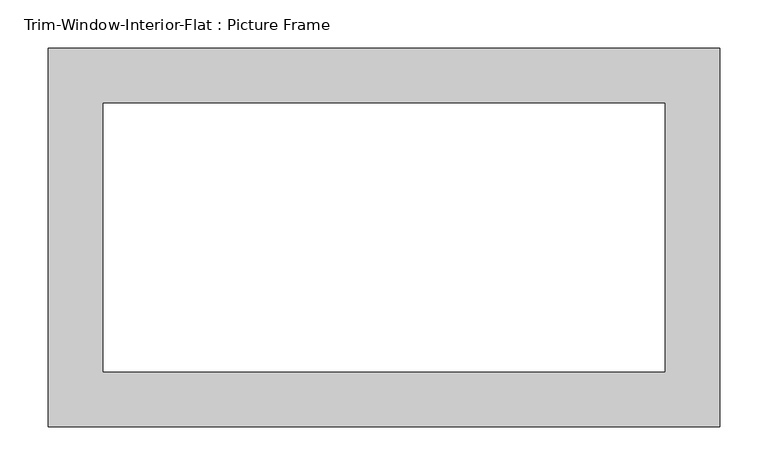
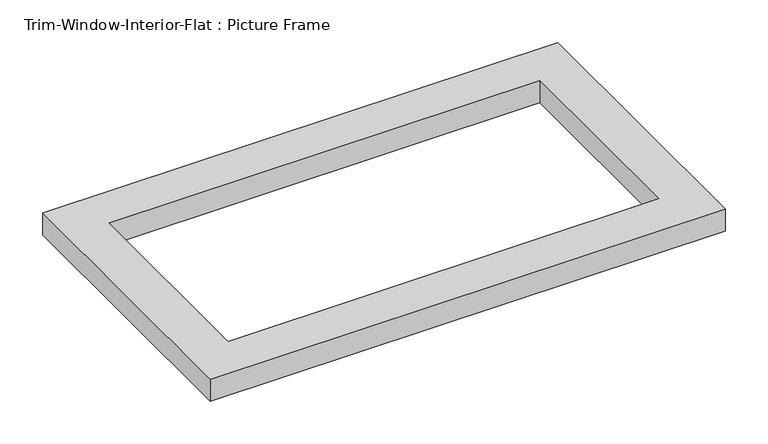
"""IFC4 building model written with IfcOpenShell, lengths in millimetres: proxy geometry, Trim-Window-Interior-Flat : Picture Frame."""

from ifc_helpers import new_model, si_unit, origin, origin_with_axes, place, context, project, spatial, polyline, outline, extrude, source, transform, mapped, element, save


def trim_window_interior_flat_picture_frame_d1e4ee8f(model_context):
    return source(origin(), model_context, "Body", "SweptSolid", [
        extrude(outline(polyline([(349.25, 44.45), (349.25, -349.25), (-349.25, -349.25), (-349.25, 44.45), (349.25, 44.45)]), holes=[polyline([(292.1, -12.7), (-292.1, -12.7), (-292.1, -292.1), (292.1, -292.1), (292.1, -12.7)])]), origin_with_axes(), (0.0, 0.0, 1.0), 31.75),
    ])


if __name__ == "__main__":
    model = new_model("IFC4")
    model_context = context("Model", 3, world=origin())
    ifc_project = project(units=[si_unit("LENGTHUNIT", "METRE", prefix="MILLI")], contexts=[model_context])
    site = spatial("IfcSite", under=ifc_project)
    building = spatial("IfcBuilding", under=site)
    placement = place(None, origin())
    trim_window_interior_flat_picture_frame_shape = trim_window_interior_flat_picture_frame_d1e4ee8f(model_context)
    element("IfcBuildingElementProxy", 1, Name="Trim-Window-Interior-Flat : Picture Frame", ObjectType="Trim-Window-Interior-Flat : Picture Frame", at=placement, inside=building, context=model_context, shape_type="MappedRepresentation", body=[
        mapped(trim_window_interior_flat_picture_frame_shape, transform((0.0, 0.0, 0.0), x_axis=(1.0, 0.0, 0.0), y_axis=(0.0, 1.0, 0.0), z_axis=(0.0, 0.0, 1.0))),
    ])
    save(model, "model.ifc")

# Revit data of these elements
# Type "Trim-Window-Interior-Flat : Picture Frame"
#   Trim Thickness_Picture Frame = 0' - 1 1/4"
#   Trim Width = 0' - 2 1/4"
#   Trim Thickness_with Sill = 0' - 0 3/4"
#   Sill Thickness = 0' - 1 1/4"
#   Opening Width [instance default] = 2' - 0"
#   Opening Height [instance default] = 3' - 0"
#   Default Elevation = 4' - 0"
#   Sill = no
#   Picture Frame = yes
#   Trim Material [instance default] = none
# Element 1 (IfcBuildingElementProxy, "Trim-Window-Interior-Flat : Picture Frame")
#   Opening Height = 1' - 0"
#   Trim Material = Wood - Stained
#   Materials on its faces: "Wood - Stained"
# Materials
#   "Wood - Stained": class "Wood", colour RGB 224 178 126, transparency 0, Cost = 0
